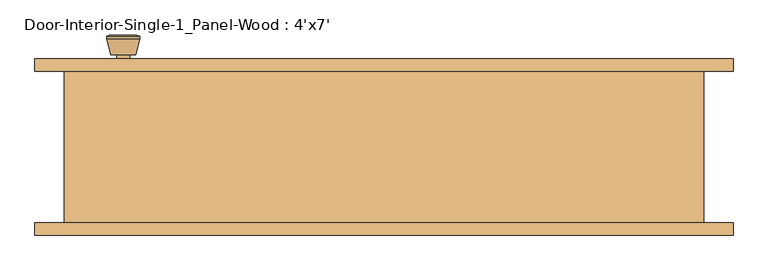
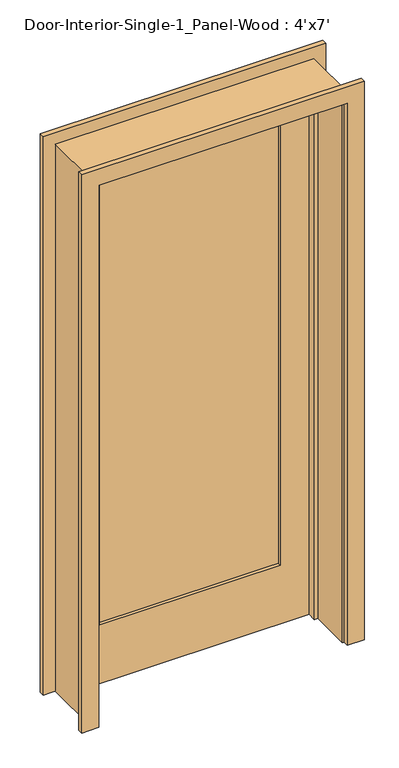
"""IFC4 building model written with IfcOpenShell, lengths in millimetres: door geometry, Door-Interior-Single-1_Panel-Wood : 4'x7'."""

from ifc_helpers import new_model, si_unit, point, frame, frame_2d, origin, place, context, project, spatial, polyline, circle_curve, trimmed, segment, composite_curve, outline, extrude, faceted_brep, source, transform, mapped, element, save
from ifc_brep_helpers import plane_surface, cylinder_surface, revolved_surface, advanced_brep


def door_interior_single_1_panel_wood_4_x7_3b97b8e7(model_context):
    return source(origin(), model_context, "Body", "SolidModel", [
        advanced_brep(
        [(-393.7, 70.2, 914.4), (-383.7, 70.2, 914.4), (-403.7, 70.2, 914.4), (-373.2241324, 21.2, 914.4), (-393.7, 21.2, 914.4), (-414.1758676, 21.2, 914.4), (-368.7, 23.0278681, 914.4), (-418.7, 23.0278681, 914.4), (-368.7, 26.4915463, 914.4), (-418.7, 26.4915463, 914.4), (-375.063764, 51.2, 914.4), (-412.336236, 51.2, 914.4), (-383.7, 51.2, 914.4), (-403.7, 51.2, 914.4)],
        [
            (0, 1),
            (1, 2, circle_curve(frame((-393.7, 70.2, 914.4), z_axis=(0.0, 1.0, 0.0), x_axis=(-1.0, 0.0, 0.0)), 10.0)),
            (2, 0),
            (2, 1, circle_curve(frame((-393.7, 70.2, 914.4), z_axis=(0.0, 1.0, 0.0), x_axis=(-1.0, 0.0, 0.0)), 10.0)),
            (3, 4),
            (4, 5),
            (5, 3, circle_curve(frame((-393.7, 21.2, 914.4), z_axis=(0.0, -1.0, 0.0), x_axis=(-1.0, 0.0, 0.0)), 20.4758676)),
            (3, 5, circle_curve(frame((-393.7, 21.2, 914.4), z_axis=(0.0, -1.0, 0.0), x_axis=(-1.0, 0.0, 0.0)), 20.4758676)),
            (6, 3),
            (5, 7),
            (7, 6, circle_curve(frame((-393.7, 23.0278681, 914.4), z_axis=(0.0, -1.0, 0.0), x_axis=(-1.0, 0.0, 0.0)), 25.0)),
            (6, 7, circle_curve(frame((-393.7, 23.0278681, 914.4), z_axis=(0.0, -1.0, 0.0), x_axis=(-1.0, 0.0, 0.0)), 25.0)),
            (8, 6),
            (7, 9),
            (9, 8, circle_curve(frame((-393.7, 26.4915463, 914.4), z_axis=(0.0, -1.0, 0.0), x_axis=(-1.0, 0.0, 0.0)), 25.0)),
            (8, 9, circle_curve(frame((-393.7, 26.4915463, 914.4), z_axis=(0.0, -1.0, 0.0), x_axis=(-1.0, 0.0, 0.0)), 25.0)),
            (10, 8),
            (9, 11),
            (11, 10, circle_curve(frame((-393.7, 51.2, 914.4), z_axis=(0.0, -1.0, 0.0), x_axis=(-1.0, 0.0, 0.0)), 18.636236)),
            (10, 11, circle_curve(frame((-393.7, 51.2, 914.4), z_axis=(0.0, -1.0, 0.0), x_axis=(-1.0, 0.0, 0.0)), 18.636236)),
            (12, 10),
            (11, 13),
            (13, 12, circle_curve(frame((-393.7, 51.2, 914.4), z_axis=(0.0, -1.0, 0.0), x_axis=(-1.0, 0.0, 0.0)), 10.0)),
            (12, 13, circle_curve(frame((-393.7, 51.2, 914.4), z_axis=(0.0, -1.0, 0.0), x_axis=(-1.0, 0.0, 0.0)), 10.0)),
            (1, 12),
            (13, 2),
        ],
        [
            plane_surface(frame((-393.7, 70.2, 914.4), z_axis=(0.0, 1.0, 0.0), x_axis=(-1.0, 0.0, 0.0))),
            plane_surface(frame((-393.7, 21.2, 914.4), z_axis=(0.0, -1.0, 0.0), x_axis=(-1.0, 0.0, 0.0))),
            revolved_surface(polyline([(-414.1758676, 21.2, 914.4), (-418.7, 23.0278681, 914.4)]), (-393.7, 70.2, 914.4), (0.0, 1.0, 0.0)),
            cylinder_surface(frame((-393.7, 70.2, 914.4), z_axis=(0.0, 1.0, 0.0), x_axis=(-1.0, 0.0, 0.0)), 25.0),
            revolved_surface(polyline([(-418.7, 26.4915463, 914.4), (-412.336236, 51.2, 914.4)]), (-393.7, 70.2, 914.4), (0.0, 1.0, 0.0)),
            plane_surface(frame((-393.7, 51.2, 914.4), z_axis=(0.0, 1.0, 0.0), x_axis=(-1.0, 0.0, 0.0))),
            cylinder_surface(frame((-393.7, 70.2, 914.4), z_axis=(0.0, 1.0, 0.0), x_axis=(-1.0, 0.0, 0.0)), 10.0),
        ],
        [
            (0, [[1, 2, 3]]),
            (0, [[-3, 4, -1]]),
            (1, [[5, 6, 7]]),
            (1, [[-6, -5, 8]]),
            (2, [[9, -7, 10, 11]]),
            (2, [[-10, -8, -9, 12]]),
            (3, [[13, -11, 14, 15]]),
            (3, [[-14, -12, -13, 16]]),
            (4, [[17, -15, 18, 19]]),
            (4, [[-18, -16, -17, 20]]),
            (5, [[21, -19, 22, 23]]),
            (5, [[-22, -20, -21, 24]]),
            (6, [[25, -23, 26, -2]]),
            (6, [[-26, -24, -25, -4]]),
        ],
    ),
        extrude(outline(composite_curve([segment(trimmed(circle_curve(frame_2d((914.4, -393.7)), 30.0), [point((914.4, -423.7))], [point((914.4, -363.7))], False, "CARTESIAN"), True, "CONTINUOUS"), segment(trimmed(circle_curve(frame_2d((914.4, -393.7)), 30.0), [point((914.4, -363.7))], [point((914.4, -423.7))], False, "CARTESIAN"), True, "CONTINUOUS")], self_intersect=False)), frame((0.0, 70.2, 0.0), z_axis=(0.0, 1.0, 0.0), x_axis=(0.0, 0.0, 1.0)), (0.0, 0.0, 1.0), 6.0),
        advanced_brep(
        [(-393.7, 117.125, 914.4), (-403.7, 117.125, 914.4), (-383.7, 117.125, 914.4), (-373.2241324, 166.125, 914.4), (-414.1758676, 166.125, 914.4), (-393.7, 166.125, 914.4), (-368.7, 164.2971319, 914.4), (-418.7, 164.2971319, 914.4), (-368.7, 160.8334537, 914.4), (-418.7, 160.8334537, 914.4), (-375.063764, 136.125, 914.4), (-412.336236, 136.125, 914.4), (-383.7, 136.125, 914.4), (-403.7, 136.125, 914.4)],
        [
            (0, 1),
            (1, 2, circle_curve(frame((-393.7, 117.125, 914.4), z_axis=(0.0, -1.0, 0.0), x_axis=(-1.0, 0.0, 0.0)), 10.0)),
            (2, 0),
            (2, 1, circle_curve(frame((-393.7, 117.125, 914.4), z_axis=(0.0, -1.0, 0.0), x_axis=(-1.0, 0.0, 0.0)), 10.0)),
            (3, 4, circle_curve(frame((-393.7, 166.125, 914.4), z_axis=(0.0, 1.0, 0.0), x_axis=(-1.0, 0.0, 0.0)), 20.4758676)),
            (4, 5),
            (5, 3),
            (4, 3, circle_curve(frame((-393.7, 166.125, 914.4), z_axis=(0.0, 1.0, 0.0), x_axis=(-1.0, 0.0, 0.0)), 20.4758676)),
            (6, 7, circle_curve(frame((-393.7, 164.2971319, 914.4), z_axis=(0.0, 1.0, 0.0), x_axis=(-1.0, 0.0, 0.0)), 25.0)),
            (7, 4),
            (3, 6),
            (7, 6, circle_curve(frame((-393.7, 164.2971319, 914.4), z_axis=(0.0, 1.0, 0.0), x_axis=(-1.0, 0.0, 0.0)), 25.0)),
            (8, 9, circle_curve(frame((-393.7, 160.8334537, 914.4), z_axis=(0.0, 1.0, 0.0), x_axis=(-1.0, 0.0, 0.0)), 25.0)),
            (9, 7),
            (6, 8),
            (9, 8, circle_curve(frame((-393.7, 160.8334537, 914.4), z_axis=(0.0, 1.0, 0.0), x_axis=(-1.0, 0.0, 0.0)), 25.0)),
            (10, 11, circle_curve(frame((-393.7, 136.125, 914.4), z_axis=(0.0, 1.0, 0.0), x_axis=(-1.0, 0.0, 0.0)), 18.636236)),
            (11, 9),
            (8, 10),
            (11, 10, circle_curve(frame((-393.7, 136.125, 914.4), z_axis=(0.0, 1.0, 0.0), x_axis=(-1.0, 0.0, 0.0)), 18.636236)),
            (12, 13, circle_curve(frame((-393.7, 136.125, 914.4), z_axis=(0.0, 1.0, 0.0), x_axis=(-1.0, 0.0, 0.0)), 10.0)),
            (13, 11),
            (10, 12),
            (13, 12, circle_curve(frame((-393.7, 136.125, 914.4), z_axis=(0.0, 1.0, 0.0), x_axis=(-1.0, 0.0, 0.0)), 10.0)),
            (1, 13),
            (12, 2),
        ],
        [
            plane_surface(frame((-393.7, 117.125, 914.4), z_axis=(0.0, -1.0, 0.0), x_axis=(-1.0, 0.0, 0.0))),
            plane_surface(frame((-393.7, 166.125, 914.4), z_axis=(0.0, 1.0, 0.0), x_axis=(-1.0, 0.0, 0.0))),
            revolved_surface(polyline([(-414.1758676, 166.125, 914.4), (-418.7, 164.2971319, 914.4)]), (-393.7, 117.125, 914.4), (0.0, -1.0, 0.0)),
            cylinder_surface(frame((-393.7, 117.125, 914.4), z_axis=(0.0, -1.0, 0.0), x_axis=(-1.0, 0.0, 0.0)), 25.0),
            revolved_surface(polyline([(-418.7, 160.8334537, 914.4), (-412.336236, 136.125, 914.4)]), (-393.7, 117.125, 914.4), (0.0, -1.0, 0.0)),
            plane_surface(frame((-393.7, 136.125, 914.4), z_axis=(0.0, -1.0, 0.0), x_axis=(-1.0, 0.0, 0.0))),
            cylinder_surface(frame((-393.7, 117.125, 914.4), z_axis=(0.0, -1.0, 0.0), x_axis=(-1.0, 0.0, 0.0)), 10.0),
        ],
        [
            (0, [[1, 2, 3]]),
            (0, [[-3, 4, -1]]),
            (1, [[5, 6, 7]]),
            (1, [[8, -7, -6]]),
            (2, [[9, 10, -5, 11]]),
            (2, [[12, -11, -8, -10]]),
            (3, [[13, 14, -9, 15]]),
            (3, [[16, -15, -12, -14]]),
            (4, [[17, 18, -13, 19]]),
            (4, [[20, -19, -16, -18]]),
            (5, [[21, 22, -17, 23]]),
            (5, [[24, -23, -20, -22]]),
            (6, [[-2, 25, -21, 26]]),
            (6, [[-4, -26, -24, -25]]),
        ],
    ),
        extrude(outline(composite_curve([segment(trimmed(circle_curve(frame_2d((914.4, -393.7)), 30.0), [point((914.4, -423.7))], [point((914.4, -363.7))], False, "CARTESIAN"), True, "CONTINUOUS"), segment(trimmed(circle_curve(frame_2d((914.4, -393.7)), 30.0), [point((914.4, -363.7))], [point((914.4, -423.7))], False, "CARTESIAN"), True, "CONTINUOUS")], self_intersect=False)), frame((0.0, 111.125, 0.0), z_axis=(0.0, 1.0, 0.0), x_axis=(0.0, 0.0, 1.0)), (0.0, 0.0, 1.0), 6.0),
        faceted_brep([(482.6, 111.125, 0.0), (482.6, -117.475, 0.0), (457.2, -117.475, 0.0), (457.2, 41.275, 0.0), (444.5, 41.275, 0.0), (444.5, 76.2, 0.0), (457.2, 76.2, 0.0), (457.2, 111.125, 0.0), (482.6, 111.125, 2159.0), (482.6, -117.475, 2159.0), (-482.6, -117.475, 2159.0), (-482.6, -117.475, 0.0), (-457.2, -117.475, 0.0), (-457.2, -117.475, 2133.6), (457.2, -117.475, 2133.6), (457.2, 41.275, 2133.6), (-457.2, 41.275, 2133.6), (-457.2, 41.275, 0.0), (-444.5, 41.275, 0.0), (-444.5, 41.275, 2120.9), (444.5, 41.275, 2120.9), (444.5, 76.2, 2120.9), (-444.5, 76.2, 2120.9), (-444.5, 76.2, 0.0), (-457.2, 76.2, 0.0), (-457.2, 76.2, 2133.6), (457.2, 76.2, 2133.6), (457.2, 111.125, 2133.6), (-457.2, 111.125, 2133.6), (-457.2, 111.125, 0.0), (-482.6, 111.125, 0.0), (-482.6, 111.125, 2159.0)], [[[0, 1, 2, 3, 4, 5, 6, 7]], [[1, 0, 8, 9]], [[2, 1, 9, 10, 11, 12, 13, 14]], [[3, 2, 14, 15]], [[4, 3, 15, 16, 17, 18, 19, 20]], [[5, 4, 20, 21]], [[6, 5, 21, 22, 23, 24, 25, 26]], [[7, 6, 26, 27]], [[0, 7, 27, 28, 29, 30, 31, 8]], [[9, 8, 31, 10]], [[15, 14, 13, 16]], [[21, 20, 19, 22]], [[27, 26, 25, 28]], [[30, 29, 24, 23, 18, 17, 12, 11]], [[10, 31, 30, 11]], [[16, 13, 12, 17]], [[22, 19, 18, 23]], [[28, 25, 24, 29]]]),
        extrude(outline(polyline([(2133.6, -457.2), (0.0, -457.2), (0.0, 457.2), (2133.6, 457.2), (2133.6, -457.2)]), holes=[polyline([(2014.5375, -336.55), (2014.5375, 336.55), (231.775, 336.55), (231.775, -336.55), (2014.5375, -336.55)])]), frame((0.0, 76.2, 0.0), z_axis=(0.0, 1.0, 0.0), x_axis=(0.0, 0.0, 1.0)), (0.0, 0.0, 1.0), 34.925),
        extrude(outline(polyline([(336.55, 87.8416667), (-336.55, 87.8416667), (-336.55, 99.4833333), (336.55, 99.4833333), (336.55, 87.8416667)])), frame((0.0, 0.0, 231.775), z_axis=(0.0, 0.0, 1.0), x_axis=(1.0, 0.0, 0.0)), (0.0, 0.0, 1.0), 1782.7625),
        extrude(outline(polyline([(0.0, 463.55), (0.0, 527.05), (2203.45, 527.05), (2203.45, -527.05), (0.0, -527.05), (0.0, -463.55), (2139.95, -463.55), (2139.95, 463.55), (0.0, 463.55)])), frame((0.0, 111.125, 0.0), z_axis=(0.0, 1.0, 0.0), x_axis=(0.0, 0.0, 1.0)), (0.0, 0.0, 1.0), 19.05),
        extrude(outline(polyline([(0.0, 463.55), (0.0, 527.05), (2203.45, 527.05), (2203.45, -527.05), (0.0, -527.05), (0.0, -463.55), (2139.95, -463.55), (2139.95, 463.55), (0.0, 463.55)])), frame((0.0, -136.525, 0.0), z_axis=(0.0, 1.0, 0.0), x_axis=(0.0, 0.0, 1.0)), (0.0, 0.0, 1.0), 19.05),
    ])


if __name__ == "__main__":
    model = new_model("IFC4")
    model_context = context("Model", 3, world=origin())
    ifc_project = project(units=[si_unit("LENGTHUNIT", "METRE", prefix="MILLI")], contexts=[model_context])
    site = spatial("IfcSite", under=ifc_project)
    building = spatial("IfcBuilding", under=site)
    placement = place(None, origin())
    door_interior_single_1_panel_wood_4_x7_shape = door_interior_single_1_panel_wood_4_x7_3b97b8e7(model_context)
    element("IfcDoor", 1, ObjectType="Door-Interior-Single-1_Panel-Wood : 4'x7'", at=placement, inside=building, context=model_context, shape_type="MappedRepresentation", body=[
        mapped(door_interior_single_1_panel_wood_4_x7_shape, transform((0.0, 0.0, 0.0), x_axis=(1.0, 0.0, 0.0), y_axis=(0.0, 1.0, 0.0), z_axis=(0.0, 0.0, 1.0))),
    ])
    save(model, "model.ifc")

# Revit data of these elements
# Type "Door-Interior-Single-1_Panel-Wood : 4'x7'"
#   Type Mark = "9"
#   Assembly Code = "C1020300"
#   Analytic Construction = "Wooden"
#   Top Rail = 0' - 4 11/16"
#   Thickness = 0' - 1 3/8"
#   Thermal Resistance (R) = 2.5876 (h·ft²·°F)/BTU
#   Swing Angle [instance default] = 90.00°
#   Stiles = 0' - 4 3/4"
#   Rough Width = 3' - 2"
#   Rough Height = 7' - 1"
#   Height = 7' - 0"
#   Width = 3' - 0"
#   Heat Transfer Coefficient (U) = 0.3865 BTU/(h·ft²·°F)
#   Bottom Rail = 0' - 9 1/8"
#   Trim Material = Cherry
#   Panel Material = Cherry
#   Frame Material = Cherry
#   Door Handle Material = Aluminum
#   Visual Light Transmittance = 0
#   Solar Heat Gain Coefficient = 0
#   Wall Closure = (empty or 0)
#   Function = (empty or 0)
# Element 1 (IfcDoor, "Door-Interior-Single-1_Panel-Wood : 4'x7'")
#   Materials on its faces: "Cherry", "Aluminum"
# Materials
#   "Cherry": class "Wood", colour RGB 226 177 128, transparency 0, Description = "Prunus Serotina", Cost = 0
#   "Aluminum": class "Metal", colour RGB 247 247 247, transparency 0, Description = "Aluminum 6061", Cost = 0
